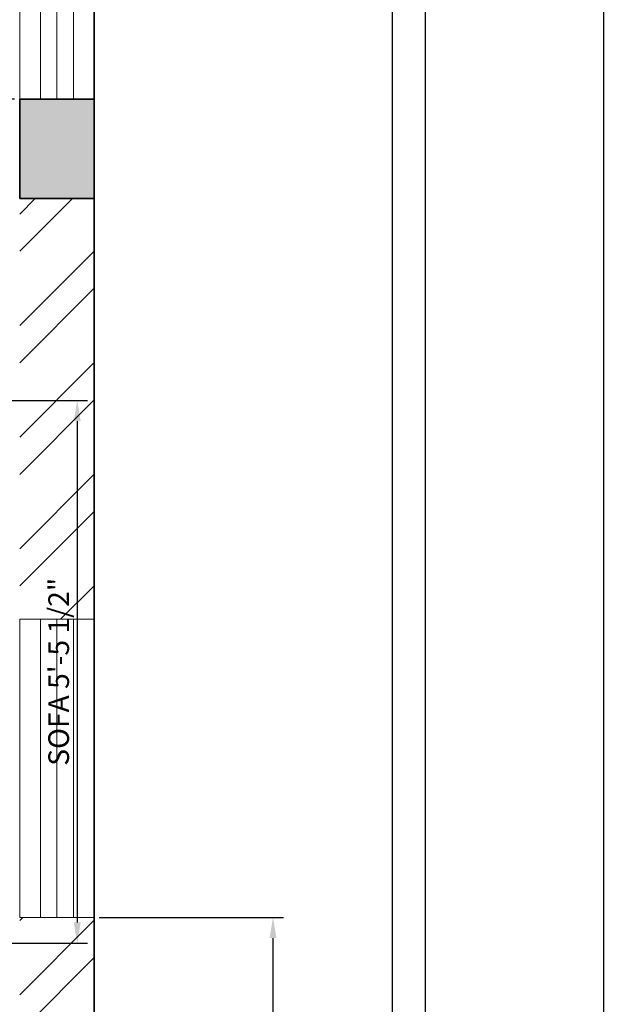
# Model space of a CAD drawing. Units: inches. Extents: x -138 to 270, y 8284 to 8764.
# Tile 9 of 10: x 198 to 270, y 8387 to 8506. Entities that reach past the tile are written whole.
import ezdxf

# ---------------------------------------------------------------- set-up
doc = ezdxf.new("R2010")
doc.units = ezdxf.units.IN
for name, color, linetype, lineweight in [('A-ANNO-DIMS', 2, 'Continuous', 18), ('C-PROP', 7, 'Continuous', 25), ('WALL', 8, 'Continuous', 35), ('WINDOW', 151, 'Continuous', 15)]:
    doc.layers.add(name, color=color, linetype=linetype, lineweight=lineweight)
doc.layers.add('A-COLS', color=252, linetype='Continuous', lineweight=35, true_color=0x939598)
doc.layers.add('A-WALL-PATT', color=32, linetype='Continuous', lineweight=9, true_color=0xbc761a)
doc.styles.get("Standard").update_dxf_attribs({"font": 'arial.ttf'})
doc.dimstyles.new('ISO-25', dxfattribs={"dimtxt": 2.5, "dimasz": 2.5, "dimexe": 1.25, "dimexo": 0.625, "dimtad": 1, "dimdec": 0, "dimlunit": 3, "dimtxsty": 'Standard', "dimcen": 2.5, "dimadec": 0, "dimazin": 0, "dimtfac": 1, "dimtdec": 0, "dimtmove": 0, "dimatfit": 3, "dimfxl": 1, "dimarcsym": 0})

# ---------------------------------------------------------------- blocks, each defined once
blk = doc.blocks.new('WINDOW-36IN')
for p, q in [((0, 6.5), (36, 6.5)), ((0, 4.5), (36, 4.5)), ((0, 2.5), (36, 2.5))]:
    blk.add_line(p, q)
blk.add_lwpolyline([(0, 0), (36, 0), (36, 9), (0, 9)], close=True)
blk = doc.blocks.new('COLUMN-9X12IN')
h = blk.add_hatch(color=256)
h.dxf.hatch_style = 1
h.paths.add_polyline_path([(9, 12), (0, 12), (0, 0), (9, 0)])
blk.add_lwpolyline([(0, 0), (9, 0), (9, 12), (0, 12)], close=True)
blk = doc.blocks.new('*D33')
at = {"layer": 'A-ANNO-DIMS', "color": 0, "lineweight": -2, "transparency": 16777216}
for p, q in [((197.45, 8532.24), (191.43, 8532.24)), ((192.68, 8498.74), (192.68, 8529.74)), ((197.45, 8496.24), (191.43, 8496.24))]:
    blk.add_line(p, q, dxfattribs=at)
at = {"layer": 'A-ANNO-DIMS', "color": 0, "transparency": 16777216}
for points in [[(192.26, 8529.74), (193.09, 8529.74), (192.68, 8532.24)], [(192.26, 8498.74), (193.09, 8498.74), (192.68, 8496.24)]]:
    blk.add_solid(points, dxfattribs=at)
at = {"layer": 'Defpoints', "color": 0, "transparency": 16777216}
for p in [(192.68, 8532.24), (198.08, 8532.24), (198.08, 8496.24)]:
    blk.add_point(p, dxfattribs=at)
at = {"layer": 'A-ANNO-DIMS', "color": 0, "transparency": 16777216, "insert": (190.77, 8514.24), "char_height": 2.5, "attachment_point": 5, "rotation": 90}
blk.add_mtext('W1 3\'-0" TYP.', dxfattribs=at)
blk = doc.blocks.new('*D43')
at = {"layer": 'A-ANNO-DIMS', "color": 0, "lineweight": -2, "transparency": 16777216}
for p, q in [((195.82, 8459.87), (206.28, 8459.87)), ((205.03, 8457.37), (205.03, 8396.81)), ((195.82, 8394.31), (206.28, 8394.31))]:
    blk.add_line(p, q, dxfattribs=at)
at = {"layer": 'A-ANNO-DIMS', "color": 0, "transparency": 16777216}
for points in [[(204.61, 8457.37), (205.45, 8457.37), (205.03, 8459.87)], [(204.61, 8396.81), (205.45, 8396.81), (205.03, 8394.31)]]:
    blk.add_solid(points, dxfattribs=at)
at = {"layer": 'Defpoints', "color": 0, "transparency": 16777216}
for p in [(195.2, 8459.87), (195.2, 8394.31), (205.03, 8394.31)]:
    blk.add_point(p, dxfattribs=at)
at = {"layer": 'A-ANNO-DIMS', "color": 0, "transparency": 16777216, "insert": (203.11, 8427.09), "char_height": 2.5, "attachment_point": 5, "rotation": 90}
blk.add_mtext('SOFA 5\'-5 1/2"', dxfattribs=at)
blk = doc.blocks.new('*D54')
at = {"layer": 'A-ANNO-DIMS', "color": 0, "lineweight": -2, "transparency": 16777216}
for p, q in [((207.7, 8699.24), (269.94, 8699.24)), ((268.69, 8349.74), (268.69, 8696.74)), ((207.7, 8347.24), (269.94, 8347.24))]:
    blk.add_line(p, q, dxfattribs=at)
at = {"layer": 'A-ANNO-DIMS', "color": 0, "transparency": 16777216}
for points in [[(268.27, 8696.74), (269.11, 8696.74), (268.69, 8699.24)], [(268.27, 8349.74), (269.11, 8349.74), (268.69, 8347.24)]]:
    blk.add_solid(points, dxfattribs=at)
at = {"layer": 'Defpoints', "color": 0, "transparency": 16777216}
for p in [(207.08, 8699.24), (268.69, 8699.24), (207.08, 8347.24)]:
    blk.add_point(p, dxfattribs=at)
at = {"layer": 'A-ANNO-DIMS', "color": 0, "transparency": 16777216, "insert": (266.79, 8523.24), "char_height": 2.5, "attachment_point": 5, "rotation": 90}
blk.add_mtext('29\'-4"', dxfattribs=at)
blk = doc.blocks.new('*D67')
at = {"layer": 'A-ANNO-DIMS', "color": 0, "lineweight": -2, "transparency": 16777216}
for p, q in [((207.7, 8397.43), (229.94, 8397.43)), ((228.69, 8394.93), (228.69, 8349.74)), ((207.7, 8347.24), (229.94, 8347.24))]:
    blk.add_line(p, q, dxfattribs=at)
at = {"layer": 'A-ANNO-DIMS', "color": 0, "transparency": 16777216}
for points in [[(228.27, 8394.93), (229.11, 8394.93), (228.69, 8397.43)], [(228.27, 8349.74), (229.11, 8349.74), (228.69, 8347.24)]]:
    blk.add_solid(points, dxfattribs=at)
at = {"layer": 'Defpoints', "color": 0, "transparency": 16777216}
for p in [(207.08, 8397.43), (207.08, 8347.24), (228.69, 8347.24)]:
    blk.add_point(p, dxfattribs=at)
at = {"layer": 'A-ANNO-DIMS', "color": 0, "transparency": 16777216, "insert": (226.81, 8372.34), "char_height": 2.5, "attachment_point": 5, "rotation": 90}
blk.add_mtext('4\'-2"', dxfattribs=at)

msp = doc.modelspace()

# ---------------------------------------------------------------- hatches: boundary and pattern name
at = {"layer": 'A-WALL-PATT'}
h = msp.add_hatch(dxfattribs=at)
h.set_pattern_fill('ANSI32', color=256)
h.paths.add_polyline_path([(115.81, 8699.24), (65.22, 8699.24), (65.22, 8690.24), (68.08, 8690.24), (68.08, 8686.36), (69.02, 8686.36), (69.02, 8686.36), (73.52, 8686.36), (74.08, 8686.36), (74.08, 8690.24), (115.81, 8690.24)])
h.paths.add_polyline_path([(169.81, 8699.24), (139.81, 8699.24), (139.81, 8690.24), (169.81, 8690.24)])
h.paths.add_polyline_path([(198.08, 8699.24), (193.81, 8699.24), (193.81, 8690.24), (198.08, 8690.24)])
h.paths.add_polyline_path([(207.08, 8648.24), (204.23, 8648.24), (204.23, 8648.24), (199.73, 8648.24), (198.08, 8648.24), (198.08, 8642.24), (150.08, 8642.24), (150.08, 8690.24), (144.08, 8690.24), (144.08, 8642.24), (74.08, 8642.24), (74.08, 8653.36), (68.08, 8653.36), (68.08, 8526.24), (68.83, 8526.24), (74.08, 8526.24), (74.08, 8630.24), (74.08, 8636.24), (98.08, 8636.24), (150.08, 8636.24), (198.08, 8636.24), (198.08, 8630.24), (198.08, 8532.24), (207.08, 8532.24)])
h.paths.add_polyline_path([(207.08, 8484.24), (198.08, 8484.24), (198.08, 8433.43), (207.08, 8433.43)])
h.paths.add_polyline_path([(198.08, 8490.24), (80.08, 8490.24), (80.08, 8484.24), (198.08, 8484.24)])
h.paths.add_polyline_path([(207.08, 8397.43), (198.08, 8397.43), (198.08, 8359.27), (207.08, 8359.27)])
h.paths.add_polyline_path([(198.08, 8356.24), (186.08, 8356.24), (186.08, 8347.24), (198.08, 8347.24)])
h.paths.add_polyline_path([(138.08, 8356.24), (128.38, 8356.24), (128.38, 8347.24), (138.08, 8347.24)])
h.paths.add_polyline_path([(92.38, 8356.24), (86.08, 8356.24), (86.08, 8347.24), (92.38, 8347.24)])

# ---------------------------------------------------------------- linework, layer by layer
at = {"layer": 'C-PROP'}
for p, q in [((247.08, 8739.24), (247.08, 8307.24)), ((243.08, 8735.24), (243.08, 8311.24))]:
    msp.add_line(p, q, dxfattribs=at)
at = {"layer": 'WALL'}
msp.add_line((207.08, 8648.24), (207.08, 8347.24), dxfattribs=at)

# ---------------------------------------------------------------- block references
at = {"layer": 'A-COLS'}
msp.add_blockref('COLUMN-9X12IN', (198.08, 8484.24), dxfattribs=at)
at = {"layer": 'WINDOW', "extrusion": (0, 0, -1), "zscale": -1, "rotation": 89.99999999999204}
for p in [(-198.08, 8496.24), (-198.08, 8397.43)]:
    msp.add_blockref('WINDOW-36IN', p, dxfattribs=at)

# ---------------------------------------------------------------- dimensions: what is measured, and where the dimension line sits
at = {"layer": 'A-ANNO-DIMS'}
for base, p1, p2, angle, picture, middle in [((268.69, 8699.24), (207.08, 8347.24), (207.08, 8699.24), 90, '*D54', (266.79, 8523.24)), ((228.69, 8347.24), (207.08, 8397.43), (207.08, 8347.24), 270, '*D67', (226.81, 8372.34))]:
    dim = msp.add_linear_dim(base=base, p1=p1, p2=p2, angle=angle, dimstyle='ISO-25', override={"dimdec": 1, "dimlfac": 1, "dimrnd": 0, "dimzin": 1, "dimdsep": 46, "dimlunit": 4, "dimfrac": 2}, dxfattribs=at)
    dim.commit()
    dim.dimension.update_dxf_attribs({"geometry": picture, "text_midpoint": middle})
for base, p1, p2, angle, text, picture, middle in [((192.68, 8532.24), (198.08, 8496.24), (198.08, 8532.24), 90, 'W1 <> TYP.', '*D33', (190.77, 8514.24)), ((205.03, 8394.31), (195.2, 8459.87), (195.2, 8394.31), 270, 'SOFA <>', '*D43', (203.11, 8427.09))]:
    dim = msp.add_linear_dim(base=base, p1=p1, p2=p2, angle=angle, text=text, dimstyle='ISO-25', override={"dimdec": 1, "dimlfac": 1, "dimrnd": 0, "dimzin": 1, "dimdsep": 46, "dimlunit": 4, "dimfrac": 2}, dxfattribs=at)
    dim.commit()
    dim.dimension.update_dxf_attribs({"geometry": picture, "text_midpoint": middle})

doc.saveas('drawing.dxf')
